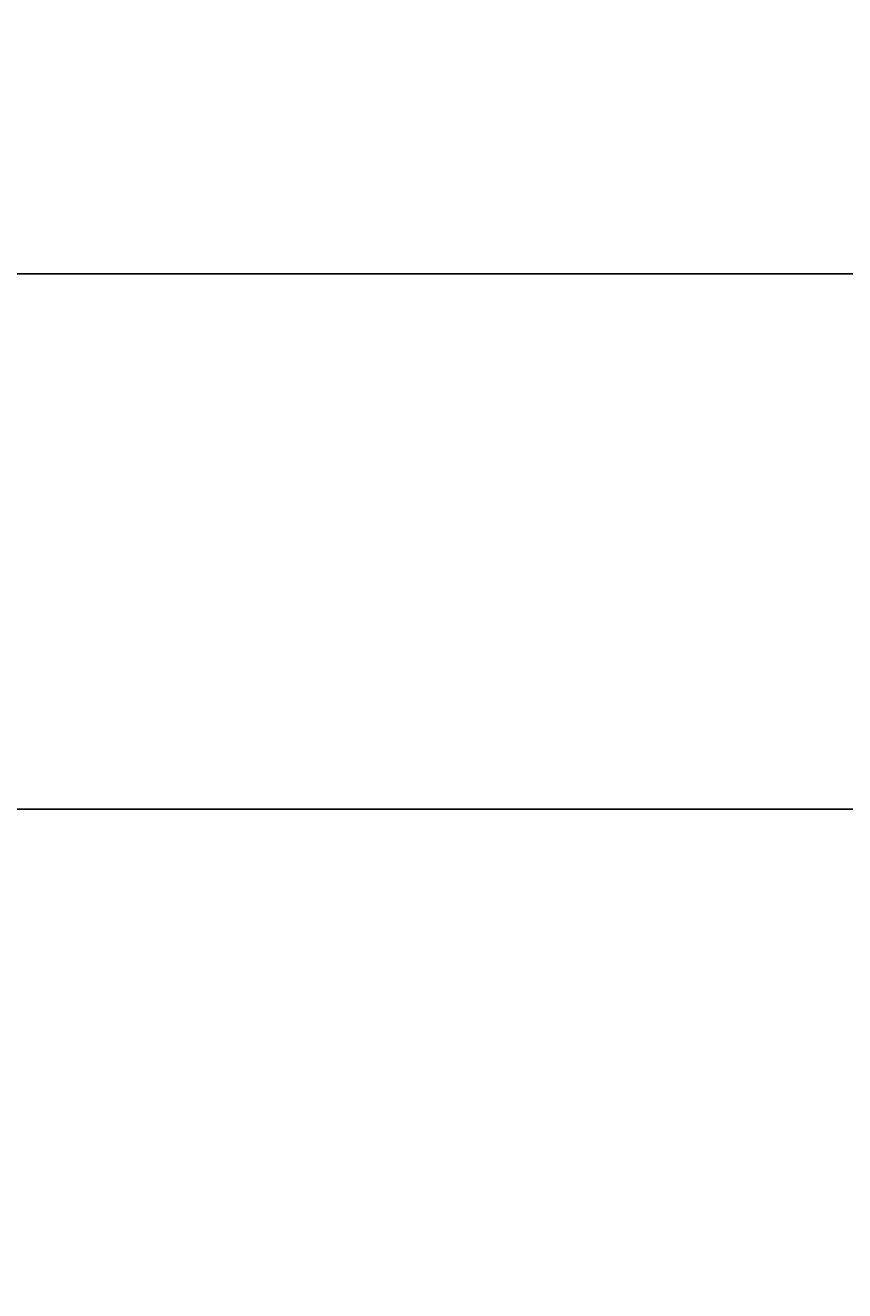
# Model space of a CAD drawing. Units: feet. Extents: x 105 to 1094, y -88 to 588.
# Tile 52 of 59: x 575 to 600, y 513 to 551. Entities that reach past the tile are written whole.
import ezdxf

# ---------------------------------------------------------------- set-up
doc = ezdxf.new("R2010")
doc.units = ezdxf.units.FT
doc.header["$MEASUREMENT"] = 0
doc.layers.add('A-ANNO-DIMS', color=2, linetype='Continuous', lineweight=18)
doc.styles.get("Standard").update_dxf_attribs({"font": 'arial.ttf'})
doc.dimstyles.get("Standard").update_dxf_attribs({"dimtxt": 0.18, "dimasz": 0.18, "dimexe": 0.18, "dimexo": 0.0625, "dimgap": 0.09, "dimtad": 0, "dimtih": 1, "dimtoh": 1, "dimdec": 4, "dimzin": 0, "dimdsep": 46, "dimtxsty": 'Standard', "dimcen": 0.09, "dimadec": 0, "dimazin": 0, "dimtfac": 1, "dimtdec": 4, "dimtofl": 0, "dimtmove": 0, "dimatfit": 3, "dimfxl": 1, "dimtolj": 1, "dimtzin": 0, "dimarcsym": 0})

# ---------------------------------------------------------------- blocks, each defined once
blk = doc.blocks.new('*D21')
at = {"layer": 'A-ANNO-DIMS', "color": 0, "lineweight": -2, "transparency": 16777216}
for p, q in [((849.626, 543.081), (105.458, 543.081)), ((105.638, 542.901), (105.638, 250.263)), ((105.638, -42.739), (105.638, 249.899)), ((849.626, -42.919), (105.458, -42.919))]:
    blk.add_line(p, q, dxfattribs=at)
at = {"layer": 'A-ANNO-DIMS', "color": 0, "transparency": 16777216}
for points in [[(105.608, 542.901), (105.668, 542.901), (105.638, 543.081)], [(105.608, -42.739), (105.668, -42.739), (105.638, -42.919)]]:
    blk.add_solid(points, dxfattribs=at)
at = {"layer": 'Defpoints', "color": 0, "transparency": 16777216}
for p in [(105.638, 543.081), (849.688, 543.081), (849.688, -42.919)]:
    blk.add_point(p, dxfattribs=at)
at = {"layer": 'A-ANNO-DIMS', "color": 0, "transparency": 16777216, "insert": (105.638, 250.081), "char_height": 0.18, "attachment_point": 5}
blk.add_mtext('\\A1;586', dxfattribs=at)
blk = doc.blocks.new('*D26')
at = {"layer": 'A-ANNO-DIMS', "color": 0, "lineweight": -2, "transparency": 16777216}
for p, q in [((552.688, 471.144), (552.688, 588.311)), ((646.688, 471.144), (646.688, 588.311)), ((552.868, 588.131), (599.47, 588.131)), ((646.508, 588.131), (599.907, 588.131))]:
    blk.add_line(p, q, dxfattribs=at)
at = {"layer": 'A-ANNO-DIMS', "color": 0, "transparency": 16777216}
for points in [[(552.868, 588.161), (552.868, 588.101), (552.688, 588.131)], [(646.508, 588.161), (646.508, 588.101), (646.688, 588.131)]]:
    blk.add_solid(points, dxfattribs=at)
at = {"layer": 'Defpoints', "color": 0, "transparency": 16777216}
for p in [(646.688, 588.131), (552.688, 471.081), (646.688, 471.081)]:
    blk.add_point(p, dxfattribs=at)
at = {"layer": 'A-ANNO-DIMS', "color": 0, "transparency": 16777216, "insert": (599.688, 588.131), "char_height": 0.18, "attachment_point": 5}
blk.add_mtext('\\A1;94', dxfattribs=at)
blk = doc.blocks.new('*D30')
at = {"layer": 'A-ANNO-DIMS', "color": 0, "lineweight": -2, "transparency": 16777216}
for p, q in [((349.751, 543.081), (1093.918, 543.081)), ((1093.738, 542.901), (1093.738, 535.263)), ((1093.738, 527.261), (1093.738, 534.899)), ((349.751, 527.081), (1093.918, 527.081))]:
    blk.add_line(p, q, dxfattribs=at)
at = {"layer": 'A-ANNO-DIMS', "color": 0, "transparency": 16777216}
for points in [[(1093.708, 542.901), (1093.768, 542.901), (1093.738, 543.081)], [(1093.708, 527.261), (1093.768, 527.261), (1093.738, 527.081)]]:
    blk.add_solid(points, dxfattribs=at)
at = {"layer": 'Defpoints', "color": 0, "transparency": 16777216}
for p in [(349.688, 543.081), (349.688, 527.081), (1093.738, 527.081)]:
    blk.add_point(p, dxfattribs=at)
at = {"layer": 'A-ANNO-DIMS', "color": 0, "transparency": 16777216, "insert": (1093.738, 535.081), "char_height": 0.18, "attachment_point": 5}
blk.add_mtext('\\A1;16', dxfattribs=at)
blk = doc.blocks.new('*D31')
at = {"layer": 'A-ANNO-DIMS', "color": 0, "lineweight": -2, "transparency": 16777216}
for p, q in [((438.751, 527.081), (1093.918, 527.081)), ((1093.738, 526.901), (1093.738, 499.263)), ((1093.738, 471.261), (1093.738, 498.899)), ((438.751, 471.081), (1093.918, 471.081))]:
    blk.add_line(p, q, dxfattribs=at)
at = {"layer": 'A-ANNO-DIMS', "color": 0, "transparency": 16777216}
for points in [[(1093.708, 526.901), (1093.768, 526.901), (1093.738, 527.081)], [(1093.708, 471.261), (1093.768, 471.261), (1093.738, 471.081)]]:
    blk.add_solid(points, dxfattribs=at)
at = {"layer": 'Defpoints', "color": 0, "transparency": 16777216}
for p in [(438.688, 527.081), (1093.738, 527.081), (438.688, 471.081)]:
    blk.add_point(p, dxfattribs=at)
at = {"layer": 'A-ANNO-DIMS', "color": 0, "transparency": 16777216, "insert": (1093.738, 499.081), "char_height": 0.18, "attachment_point": 5}
blk.add_mtext('\\A1;56', dxfattribs=at)
blk = doc.blocks.new('*D48')
at = {"layer": 'A-ANNO-DIMS', "color": 0, "lineweight": -2, "transparency": 16777216}
for p, q in [((573.483, 441.144), (573.483, 588.311)), ((633.483, 441.144), (633.483, 588.311)), ((573.663, 588.131), (603.263, 588.131)), ((633.303, 588.131), (603.702, 588.131))]:
    blk.add_line(p, q, dxfattribs=at)
at = {"layer": 'A-ANNO-DIMS', "color": 0, "transparency": 16777216}
for points in [[(573.663, 588.161), (573.663, 588.101), (573.483, 588.131)], [(633.303, 588.161), (633.303, 588.101), (633.483, 588.131)]]:
    blk.add_solid(points, dxfattribs=at)
at = {"layer": 'Defpoints', "color": 0, "transparency": 16777216}
for p in [(633.483, 588.131), (573.483, 441.081), (633.483, 441.081)]:
    blk.add_point(p, dxfattribs=at)
at = {"layer": 'A-ANNO-DIMS', "color": 0, "transparency": 16777216, "insert": (603.483, 588.131), "char_height": 0.18, "attachment_point": 5}
blk.add_mtext('\\A1;60', dxfattribs=at)

msp = doc.modelspace()

# ---------------------------------------------------------------- dimensions: what is measured, and where the dimension line sits
at = {"layer": 'A-ANNO-DIMS'}
for base, p1, p2, picture, middle in [((646.6883, 588.1312), (552.6883, 471.0812), (646.6883, 471.0812), '*D26', (599.6883, 588.1312)), ((633.4826, 588.1312), (573.4826, 441.0812), (633.4826, 441.0812), '*D48', (603.4826, 588.1312))]:
    dim = msp.add_linear_dim(base=base, p1=p1, p2=p2, dimstyle='Standard', override={"dimdec": 0, "dimlfac": 1, "dimrnd": 0, "dimzin": 0, "dimdsep": 46, "dimlunit": 2}, dxfattribs=at)
    dim.commit()
    dim.dimension.update_dxf_attribs({"geometry": picture, "text_midpoint": middle})
for base, p1, p2, picture, middle in [((105.6383, 543.0812), (849.6883, -42.9188), (849.6883, 543.0812), '*D21', (105.6383, 250.0812)), ((1093.7383, 527.0812), (349.6883, 543.0812), (349.6883, 527.0812), '*D30', (1093.7383, 535.0812)), ((1093.7383, 527.0812), (438.6883, 471.0812), (438.6883, 527.0812), '*D31', (1093.7383, 499.0812))]:
    dim = msp.add_linear_dim(base=base, p1=p1, p2=p2, angle=90, dimstyle='Standard', override={"dimdec": 0, "dimlfac": 1, "dimrnd": 0, "dimzin": 0, "dimdsep": 46, "dimlunit": 2}, dxfattribs=at)
    dim.commit()
    dim.dimension.update_dxf_attribs({"geometry": picture, "text_midpoint": middle})

doc.saveas('drawing.dxf')
